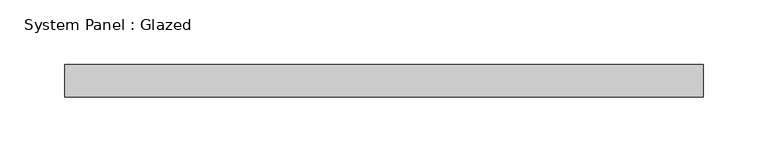
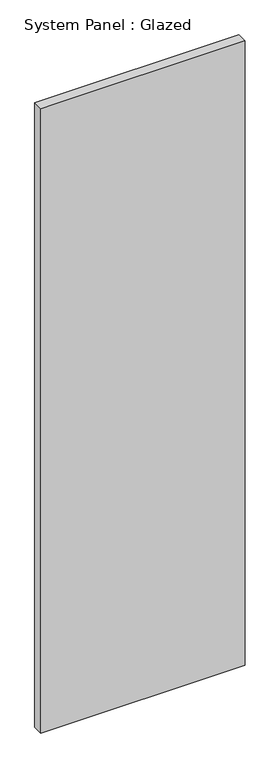
"""IFC4 building model written with IfcOpenShell, lengths in millimetres: plate geometry, System Panel : Glazed."""

from ifc_helpers import new_model, si_unit, origin, origin_with_axes, place, context, project, spatial, polyline, outline, extrude, source, transform, mapped, element, save


def system_panel_glazed_a6fbc2a7(model_context):
    return source(origin(), model_context, "Body", "SweptSolid", [
        extrude(outline(polyline([(247.65, 19.05), (-247.65, 19.05), (-247.65, 44.45), (247.65, 44.45), (247.65, 19.05)])), origin_with_axes(), (0.0, 0.0, 1.0), 1601.1374524),
    ])


if __name__ == "__main__":
    model = new_model("IFC4")
    model_context = context("Model", 3, world=origin())
    ifc_project = project(units=[si_unit("LENGTHUNIT", "METRE", prefix="MILLI")], contexts=[model_context])
    site = spatial("IfcSite", under=ifc_project)
    building = spatial("IfcBuilding", under=site)
    placement = place(None, origin())
    system_panel_glazed_shape = system_panel_glazed_a6fbc2a7(model_context)
    element("IfcPlate", 1, ObjectType="System Panel : Glazed", at=placement, inside=building, context=model_context, shape_type="MappedRepresentation", body=[
        mapped(system_panel_glazed_shape, transform((0.0, 0.0, 0.0), x_axis=(1.0, 0.0, 0.0), y_axis=(0.0, 1.0, 0.0), z_axis=(0.0, 0.0, 1.0))),
    ])
    save(model, "model.ifc")

# Revit data of these elements
# Type "System Panel : Glazed"
#   Construction Type Id = "GSP4R"
#   Analytic Construction = "1/8 in Pilkington single glazing"
#   Visual Light Transmittance = 0.9
#   Solar Heat Gain Coefficient = 0.86
#   Heat Transfer Coefficient (U) = 1.18115 BTU/(h·ft²·°F)
#   Define Thermal Properties by = 1
# Element 1 (IfcPlate, "System Panel : Glazed")
#   Materials on its faces: "Glass"
# Materials
#   "Glass": class "Glass", colour RGB 0 128 192, transparency 0.75, Description = "Soda Lime Glass", Cost = 0
